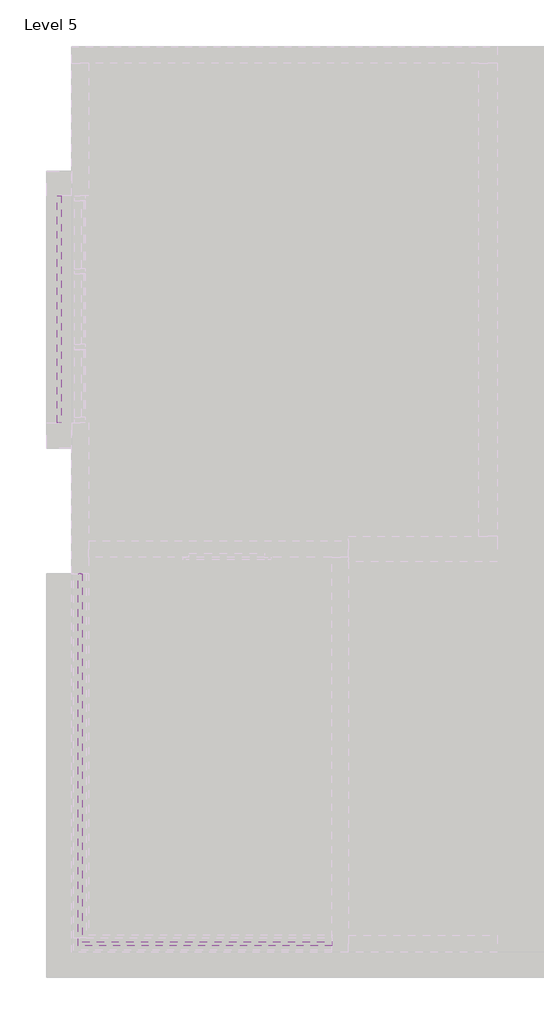
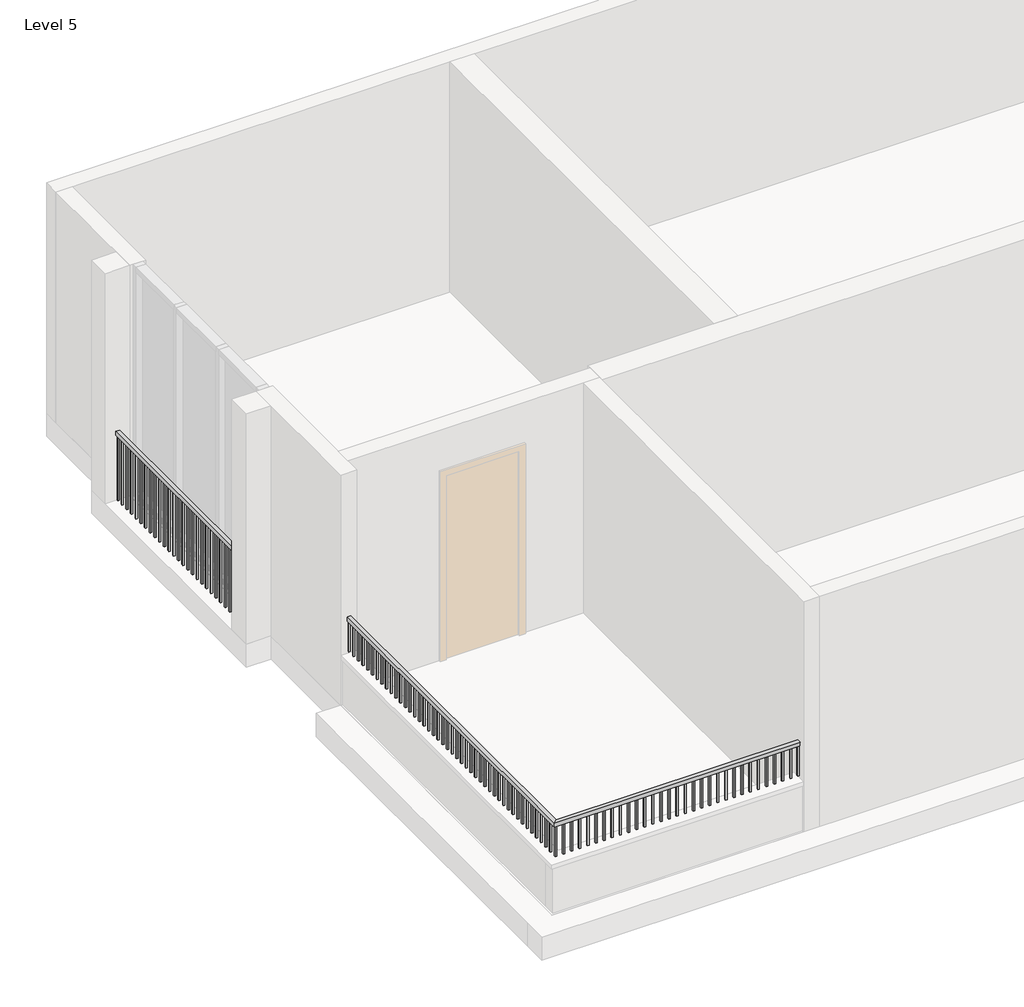
# One storey, part 2 of 2: 2 railings.
"""IFC4 building model written with IfcOpenShell, lengths in millimetres."""

from ifc_helpers import new_model, si_unit, frame, origin, place, context, project, spatial, polyline, outline, extrude, faceted_brep, element, save

model = new_model("IFC4")

# Units and contexts
model_context = context("Model", 3, world=origin())
ifc_project = project(units=[si_unit("LENGTHUNIT", "METRE", prefix="MILLI")], contexts=[model_context])

# Site, building, storey
site = spatial("IfcSite", under=ifc_project)
building = spatial("IfcBuilding", under=site)
storey = spatial("IfcBuildingStorey", under=building, Name="Level 5", Elevation=12192.0)

# Railings
placement = place(None, origin())
element("IfcRailing", 1, ObjectType="Handrail - Rectangular", at=placement, inside=storey, context=model_context, shape_type="SolidModel", body=[
    faceted_brep([(-15179.2169582, -9411.0617616, 14554.2), (-15179.2169582, -9411.0617616, 14503.4), (-15179.2169582, -9360.2617616, 14503.4), (-15179.2169582, -9360.2617616, 14554.2), (-18252.6169582, -9411.0617616, 14554.2), (-18252.6169582, -9411.0617616, 14503.4), (-18201.8169582, -9360.2617616, 14503.4), (-18201.8169582, -9360.2617616, 14554.2), (-18252.6169582, -4908.9117616, 14554.2), (-18201.8169582, -4908.9117616, 14554.2), (-18201.8169582, -4908.9117616, 14503.4), (-18252.6169582, -4908.9117616, 14503.4)], [[[0, 1, 2, 3]], [[1, 0, 4, 5]], [[2, 1, 5, 6]], [[3, 2, 6, 7]], [[0, 3, 7, 4]], [[8, 9, 10, 11]], [[5, 4, 8, 11]], [[6, 5, 11, 10]], [[7, 6, 10, 9]], [[4, 7, 9, 8]]]),
    extrude(outline(polyline([(-18217.6919582, -4924.7867616), (-18236.7419582, -4924.7867616), (-18236.7419582, -4905.7367616), (-18217.6919582, -4905.7367616), (-18217.6919582, -4924.7867616)])), frame((0.0, 0.0, 14097.0), z_axis=(0.0, 0.0, 1.0), x_axis=(1.0, 0.0, 0.0)), (0.0, 0.0, 1.0), 406.4),
    extrude(outline(polyline([(-18217.6919582, -5026.3867616), (-18236.7419582, -5026.3867616), (-18236.7419582, -5007.3367616), (-18217.6919582, -5007.3367616), (-18217.6919582, -5026.3867616)])), frame((0.0, 0.0, 14097.0), z_axis=(0.0, 0.0, 1.0), x_axis=(1.0, 0.0, 0.0)), (0.0, 0.0, 1.0), 406.4),
    extrude(outline(polyline([(-18217.6919582, -5127.9867616), (-18236.7419582, -5127.9867616), (-18236.7419582, -5108.9367616), (-18217.6919582, -5108.9367616), (-18217.6919582, -5127.9867616)])), frame((0.0, 0.0, 14097.0), z_axis=(0.0, 0.0, 1.0), x_axis=(1.0, 0.0, 0.0)), (0.0, 0.0, 1.0), 406.4),
    extrude(outline(polyline([(-18217.6919582, -5229.5867616), (-18236.7419582, -5229.5867616), (-18236.7419582, -5210.5367616), (-18217.6919582, -5210.5367616), (-18217.6919582, -5229.5867616)])), frame((0.0, 0.0, 14097.0), z_axis=(0.0, 0.0, 1.0), x_axis=(1.0, 0.0, 0.0)), (0.0, 0.0, 1.0), 406.4),
    extrude(outline(polyline([(-18217.6919582, -5331.1867616), (-18236.7419582, -5331.1867616), (-18236.7419582, -5312.1367616), (-18217.6919582, -5312.1367616), (-18217.6919582, -5331.1867616)])), frame((0.0, 0.0, 14097.0), z_axis=(0.0, 0.0, 1.0), x_axis=(1.0, 0.0, 0.0)), (0.0, 0.0, 1.0), 406.4),
    extrude(outline(polyline([(-18217.6919582, -5432.7867616), (-18236.7419582, -5432.7867616), (-18236.7419582, -5413.7367616), (-18217.6919582, -5413.7367616), (-18217.6919582, -5432.7867616)])), frame((0.0, 0.0, 14097.0), z_axis=(0.0, 0.0, 1.0), x_axis=(1.0, 0.0, 0.0)), (0.0, 0.0, 1.0), 406.4),
    extrude(outline(polyline([(-18217.6919582, -5534.3867616), (-18236.7419582, -5534.3867616), (-18236.7419582, -5515.3367616), (-18217.6919582, -5515.3367616), (-18217.6919582, -5534.3867616)])), frame((0.0, 0.0, 14097.0), z_axis=(0.0, 0.0, 1.0), x_axis=(1.0, 0.0, 0.0)), (0.0, 0.0, 1.0), 406.4),
    extrude(outline(polyline([(-18217.6919582, -5635.9867616), (-18236.7419582, -5635.9867616), (-18236.7419582, -5616.9367616), (-18217.6919582, -5616.9367616), (-18217.6919582, -5635.9867616)])), frame((0.0, 0.0, 14097.0), z_axis=(0.0, 0.0, 1.0), x_axis=(1.0, 0.0, 0.0)), (0.0, 0.0, 1.0), 406.4),
    extrude(outline(polyline([(-18217.6919582, -5737.5867616), (-18236.7419582, -5737.5867616), (-18236.7419582, -5718.5367616), (-18217.6919582, -5718.5367616), (-18217.6919582, -5737.5867616)])), frame((0.0, 0.0, 14097.0), z_axis=(0.0, 0.0, 1.0), x_axis=(1.0, 0.0, 0.0)), (0.0, 0.0, 1.0), 406.4),
    extrude(outline(polyline([(-18217.6919582, -5839.1867616), (-18236.7419582, -5839.1867616), (-18236.7419582, -5820.1367616), (-18217.6919582, -5820.1367616), (-18217.6919582, -5839.1867616)])), frame((0.0, 0.0, 14097.0), z_axis=(0.0, 0.0, 1.0), x_axis=(1.0, 0.0, 0.0)), (0.0, 0.0, 1.0), 406.4),
    extrude(outline(polyline([(-18217.6919582, -5940.7867616), (-18236.7419582, -5940.7867616), (-18236.7419582, -5921.7367616), (-18217.6919582, -5921.7367616), (-18217.6919582, -5940.7867616)])), frame((0.0, 0.0, 14097.0), z_axis=(0.0, 0.0, 1.0), x_axis=(1.0, 0.0, 0.0)), (0.0, 0.0, 1.0), 406.4),
    extrude(outline(polyline([(-18217.6919582, -6042.3867616), (-18236.7419582, -6042.3867616), (-18236.7419582, -6023.3367616), (-18217.6919582, -6023.3367616), (-18217.6919582, -6042.3867616)])), frame((0.0, 0.0, 14097.0), z_axis=(0.0, 0.0, 1.0), x_axis=(1.0, 0.0, 0.0)), (0.0, 0.0, 1.0), 406.4),
    extrude(outline(polyline([(-18217.6919582, -6143.9867616), (-18236.7419582, -6143.9867616), (-18236.7419582, -6124.9367616), (-18217.6919582, -6124.9367616), (-18217.6919582, -6143.9867616)])), frame((0.0, 0.0, 14097.0), z_axis=(0.0, 0.0, 1.0), x_axis=(1.0, 0.0, 0.0)), (0.0, 0.0, 1.0), 406.4),
    extrude(outline(polyline([(-18217.6919582, -6245.5867616), (-18236.7419582, -6245.5867616), (-18236.7419582, -6226.5367616), (-18217.6919582, -6226.5367616), (-18217.6919582, -6245.5867616)])), frame((0.0, 0.0, 14097.0), z_axis=(0.0, 0.0, 1.0), x_axis=(1.0, 0.0, 0.0)), (0.0, 0.0, 1.0), 406.4),
    extrude(outline(polyline([(-18217.6919582, -6347.1867616), (-18236.7419582, -6347.1867616), (-18236.7419582, -6328.1367616), (-18217.6919582, -6328.1367616), (-18217.6919582, -6347.1867616)])), frame((0.0, 0.0, 14097.0), z_axis=(0.0, 0.0, 1.0), x_axis=(1.0, 0.0, 0.0)), (0.0, 0.0, 1.0), 406.4),
    extrude(outline(polyline([(-18217.6919582, -6448.7867616), (-18236.7419582, -6448.7867616), (-18236.7419582, -6429.7367616), (-18217.6919582, -6429.7367616), (-18217.6919582, -6448.7867616)])), frame((0.0, 0.0, 14097.0), z_axis=(0.0, 0.0, 1.0), x_axis=(1.0, 0.0, 0.0)), (0.0, 0.0, 1.0), 406.4),
    extrude(outline(polyline([(-18217.6919582, -6550.3867616), (-18236.7419582, -6550.3867616), (-18236.7419582, -6531.3367616), (-18217.6919582, -6531.3367616), (-18217.6919582, -6550.3867616)])), frame((0.0, 0.0, 14097.0), z_axis=(0.0, 0.0, 1.0), x_axis=(1.0, 0.0, 0.0)), (0.0, 0.0, 1.0), 406.4),
    extrude(outline(polyline([(-18217.6919582, -6651.9867616), (-18236.7419582, -6651.9867616), (-18236.7419582, -6632.9367616), (-18217.6919582, -6632.9367616), (-18217.6919582, -6651.9867616)])), frame((0.0, 0.0, 14097.0), z_axis=(0.0, 0.0, 1.0), x_axis=(1.0, 0.0, 0.0)), (0.0, 0.0, 1.0), 406.4),
    extrude(outline(polyline([(-18217.6919582, -6753.5867616), (-18236.7419582, -6753.5867616), (-18236.7419582, -6734.5367616), (-18217.6919582, -6734.5367616), (-18217.6919582, -6753.5867616)])), frame((0.0, 0.0, 14097.0), z_axis=(0.0, 0.0, 1.0), x_axis=(1.0, 0.0, 0.0)), (0.0, 0.0, 1.0), 406.4),
    extrude(outline(polyline([(-18217.6919582, -6855.1867616), (-18236.7419582, -6855.1867616), (-18236.7419582, -6836.1367616), (-18217.6919582, -6836.1367616), (-18217.6919582, -6855.1867616)])), frame((0.0, 0.0, 14097.0), z_axis=(0.0, 0.0, 1.0), x_axis=(1.0, 0.0, 0.0)), (0.0, 0.0, 1.0), 406.4),
    extrude(outline(polyline([(-18217.6919582, -6956.7867616), (-18236.7419582, -6956.7867616), (-18236.7419582, -6937.7367616), (-18217.6919582, -6937.7367616), (-18217.6919582, -6956.7867616)])), frame((0.0, 0.0, 14097.0), z_axis=(0.0, 0.0, 1.0), x_axis=(1.0, 0.0, 0.0)), (0.0, 0.0, 1.0), 406.4),
    extrude(outline(polyline([(-18217.6919582, -7058.3867616), (-18236.7419582, -7058.3867616), (-18236.7419582, -7039.3367616), (-18217.6919582, -7039.3367616), (-18217.6919582, -7058.3867616)])), frame((0.0, 0.0, 14097.0), z_axis=(0.0, 0.0, 1.0), x_axis=(1.0, 0.0, 0.0)), (0.0, 0.0, 1.0), 406.4),
    extrude(outline(polyline([(-18217.6919582, -7159.9867616), (-18236.7419582, -7159.9867616), (-18236.7419582, -7140.9367616), (-18217.6919582, -7140.9367616), (-18217.6919582, -7159.9867616)])), frame((0.0, 0.0, 14097.0), z_axis=(0.0, 0.0, 1.0), x_axis=(1.0, 0.0, 0.0)), (0.0, 0.0, 1.0), 406.4),
    extrude(outline(polyline([(-18217.6919582, -7261.5867616), (-18236.7419582, -7261.5867616), (-18236.7419582, -7242.5367616), (-18217.6919582, -7242.5367616), (-18217.6919582, -7261.5867616)])), frame((0.0, 0.0, 14097.0), z_axis=(0.0, 0.0, 1.0), x_axis=(1.0, 0.0, 0.0)), (0.0, 0.0, 1.0), 406.4),
    extrude(outline(polyline([(-18217.6919582, -7363.1867616), (-18236.7419582, -7363.1867616), (-18236.7419582, -7344.1367616), (-18217.6919582, -7344.1367616), (-18217.6919582, -7363.1867616)])), frame((0.0, 0.0, 14097.0), z_axis=(0.0, 0.0, 1.0), x_axis=(1.0, 0.0, 0.0)), (0.0, 0.0, 1.0), 406.4),
    extrude(outline(polyline([(-18217.6919582, -7464.7867616), (-18236.7419582, -7464.7867616), (-18236.7419582, -7445.7367616), (-18217.6919582, -7445.7367616), (-18217.6919582, -7464.7867616)])), frame((0.0, 0.0, 14097.0), z_axis=(0.0, 0.0, 1.0), x_axis=(1.0, 0.0, 0.0)), (0.0, 0.0, 1.0), 406.4),
    extrude(outline(polyline([(-18217.6919582, -7566.3867616), (-18236.7419582, -7566.3867616), (-18236.7419582, -7547.3367616), (-18217.6919582, -7547.3367616), (-18217.6919582, -7566.3867616)])), frame((0.0, 0.0, 14097.0), z_axis=(0.0, 0.0, 1.0), x_axis=(1.0, 0.0, 0.0)), (0.0, 0.0, 1.0), 406.4),
    extrude(outline(polyline([(-18217.6919582, -7667.9867616), (-18236.7419582, -7667.9867616), (-18236.7419582, -7648.9367616), (-18217.6919582, -7648.9367616), (-18217.6919582, -7667.9867616)])), frame((0.0, 0.0, 14097.0), z_axis=(0.0, 0.0, 1.0), x_axis=(1.0, 0.0, 0.0)), (0.0, 0.0, 1.0), 406.4),
    extrude(outline(polyline([(-18217.6919582, -7769.5867616), (-18236.7419582, -7769.5867616), (-18236.7419582, -7750.5367616), (-18217.6919582, -7750.5367616), (-18217.6919582, -7769.5867616)])), frame((0.0, 0.0, 14097.0), z_axis=(0.0, 0.0, 1.0), x_axis=(1.0, 0.0, 0.0)), (0.0, 0.0, 1.0), 406.4),
    extrude(outline(polyline([(-18217.6919582, -7871.1867616), (-18236.7419582, -7871.1867616), (-18236.7419582, -7852.1367616), (-18217.6919582, -7852.1367616), (-18217.6919582, -7871.1867616)])), frame((0.0, 0.0, 14097.0), z_axis=(0.0, 0.0, 1.0), x_axis=(1.0, 0.0, 0.0)), (0.0, 0.0, 1.0), 406.4),
    extrude(outline(polyline([(-18217.6919582, -7972.7867616), (-18236.7419582, -7972.7867616), (-18236.7419582, -7953.7367616), (-18217.6919582, -7953.7367616), (-18217.6919582, -7972.7867616)])), frame((0.0, 0.0, 14097.0), z_axis=(0.0, 0.0, 1.0), x_axis=(1.0, 0.0, 0.0)), (0.0, 0.0, 1.0), 406.4),
    extrude(outline(polyline([(-18217.6919582, -8074.3867616), (-18236.7419582, -8074.3867616), (-18236.7419582, -8055.3367616), (-18217.6919582, -8055.3367616), (-18217.6919582, -8074.3867616)])), frame((0.0, 0.0, 14097.0), z_axis=(0.0, 0.0, 1.0), x_axis=(1.0, 0.0, 0.0)), (0.0, 0.0, 1.0), 406.4),
    extrude(outline(polyline([(-18217.6919582, -8175.9867616), (-18236.7419582, -8175.9867616), (-18236.7419582, -8156.9367616), (-18217.6919582, -8156.9367616), (-18217.6919582, -8175.9867616)])), frame((0.0, 0.0, 14097.0), z_axis=(0.0, 0.0, 1.0), x_axis=(1.0, 0.0, 0.0)), (0.0, 0.0, 1.0), 406.4),
    extrude(outline(polyline([(-18217.6919582, -8277.5867616), (-18236.7419582, -8277.5867616), (-18236.7419582, -8258.5367616), (-18217.6919582, -8258.5367616), (-18217.6919582, -8277.5867616)])), frame((0.0, 0.0, 14097.0), z_axis=(0.0, 0.0, 1.0), x_axis=(1.0, 0.0, 0.0)), (0.0, 0.0, 1.0), 406.4),
    extrude(outline(polyline([(-18217.6919582, -8379.1867616), (-18236.7419582, -8379.1867616), (-18236.7419582, -8360.1367616), (-18217.6919582, -8360.1367616), (-18217.6919582, -8379.1867616)])), frame((0.0, 0.0, 14097.0), z_axis=(0.0, 0.0, 1.0), x_axis=(1.0, 0.0, 0.0)), (0.0, 0.0, 1.0), 406.4),
    extrude(outline(polyline([(-18217.6919582, -8480.7867616), (-18236.7419582, -8480.7867616), (-18236.7419582, -8461.7367616), (-18217.6919582, -8461.7367616), (-18217.6919582, -8480.7867616)])), frame((0.0, 0.0, 14097.0), z_axis=(0.0, 0.0, 1.0), x_axis=(1.0, 0.0, 0.0)), (0.0, 0.0, 1.0), 406.4),
    extrude(outline(polyline([(-18217.6919582, -8582.3867616), (-18236.7419582, -8582.3867616), (-18236.7419582, -8563.3367616), (-18217.6919582, -8563.3367616), (-18217.6919582, -8582.3867616)])), frame((0.0, 0.0, 14097.0), z_axis=(0.0, 0.0, 1.0), x_axis=(1.0, 0.0, 0.0)), (0.0, 0.0, 1.0), 406.4),
    extrude(outline(polyline([(-18217.6919582, -8683.9867616), (-18236.7419582, -8683.9867616), (-18236.7419582, -8664.9367616), (-18217.6919582, -8664.9367616), (-18217.6919582, -8683.9867616)])), frame((0.0, 0.0, 14097.0), z_axis=(0.0, 0.0, 1.0), x_axis=(1.0, 0.0, 0.0)), (0.0, 0.0, 1.0), 406.4),
    extrude(outline(polyline([(-18217.6919582, -8785.5867616), (-18236.7419582, -8785.5867616), (-18236.7419582, -8766.5367616), (-18217.6919582, -8766.5367616), (-18217.6919582, -8785.5867616)])), frame((0.0, 0.0, 14097.0), z_axis=(0.0, 0.0, 1.0), x_axis=(1.0, 0.0, 0.0)), (0.0, 0.0, 1.0), 406.4),
    extrude(outline(polyline([(-18217.6919582, -8887.1867616), (-18236.7419582, -8887.1867616), (-18236.7419582, -8868.1367616), (-18217.6919582, -8868.1367616), (-18217.6919582, -8887.1867616)])), frame((0.0, 0.0, 14097.0), z_axis=(0.0, 0.0, 1.0), x_axis=(1.0, 0.0, 0.0)), (0.0, 0.0, 1.0), 406.4),
    extrude(outline(polyline([(-18217.6919582, -8988.7867616), (-18236.7419582, -8988.7867616), (-18236.7419582, -8969.7367616), (-18217.6919582, -8969.7367616), (-18217.6919582, -8988.7867616)])), frame((0.0, 0.0, 14097.0), z_axis=(0.0, 0.0, 1.0), x_axis=(1.0, 0.0, 0.0)), (0.0, 0.0, 1.0), 406.4),
    extrude(outline(polyline([(-18217.6919582, -9090.3867616), (-18236.7419582, -9090.3867616), (-18236.7419582, -9071.3367616), (-18217.6919582, -9071.3367616), (-18217.6919582, -9090.3867616)])), frame((0.0, 0.0, 14097.0), z_axis=(0.0, 0.0, 1.0), x_axis=(1.0, 0.0, 0.0)), (0.0, 0.0, 1.0), 406.4),
    extrude(outline(polyline([(-18217.6919582, -9191.9867616), (-18236.7419582, -9191.9867616), (-18236.7419582, -9172.9367616), (-18217.6919582, -9172.9367616), (-18217.6919582, -9191.9867616)])), frame((0.0, 0.0, 14097.0), z_axis=(0.0, 0.0, 1.0), x_axis=(1.0, 0.0, 0.0)), (0.0, 0.0, 1.0), 406.4),
    extrude(outline(polyline([(-18217.6919582, -9293.5867616), (-18236.7419582, -9293.5867616), (-18236.7419582, -9274.5367616), (-18217.6919582, -9274.5367616), (-18217.6919582, -9293.5867616)])), frame((0.0, 0.0, 14097.0), z_axis=(0.0, 0.0, 1.0), x_axis=(1.0, 0.0, 0.0)), (0.0, 0.0, 1.0), 406.4),
    extrude(outline(polyline([(-18116.0919582, -9376.1367616), (-18116.0919582, -9395.1867616), (-18135.1419582, -9395.1867616), (-18135.1419582, -9376.1367616), (-18116.0919582, -9376.1367616)])), frame((0.0, 0.0, 14097.0), z_axis=(0.0, 0.0, 1.0), x_axis=(1.0, 0.0, 0.0)), (0.0, 0.0, 1.0), 406.4),
    extrude(outline(polyline([(-18014.4919582, -9376.1367616), (-18014.4919582, -9395.1867616), (-18033.5419582, -9395.1867616), (-18033.5419582, -9376.1367616), (-18014.4919582, -9376.1367616)])), frame((0.0, 0.0, 14097.0), z_axis=(0.0, 0.0, 1.0), x_axis=(1.0, 0.0, 0.0)), (0.0, 0.0, 1.0), 406.4),
    extrude(outline(polyline([(-17912.8919582, -9376.1367616), (-17912.8919582, -9395.1867616), (-17931.9419582, -9395.1867616), (-17931.9419582, -9376.1367616), (-17912.8919582, -9376.1367616)])), frame((0.0, 0.0, 14097.0), z_axis=(0.0, 0.0, 1.0), x_axis=(1.0, 0.0, 0.0)), (0.0, 0.0, 1.0), 406.4),
    extrude(outline(polyline([(-17811.2919582, -9376.1367616), (-17811.2919582, -9395.1867616), (-17830.3419582, -9395.1867616), (-17830.3419582, -9376.1367616), (-17811.2919582, -9376.1367616)])), frame((0.0, 0.0, 14097.0), z_axis=(0.0, 0.0, 1.0), x_axis=(1.0, 0.0, 0.0)), (0.0, 0.0, 1.0), 406.4),
    extrude(outline(polyline([(-17709.6919582, -9376.1367616), (-17709.6919582, -9395.1867616), (-17728.7419582, -9395.1867616), (-17728.7419582, -9376.1367616), (-17709.6919582, -9376.1367616)])), frame((0.0, 0.0, 14097.0), z_axis=(0.0, 0.0, 1.0), x_axis=(1.0, 0.0, 0.0)), (0.0, 0.0, 1.0), 406.4),
    extrude(outline(polyline([(-17608.0919582, -9376.1367616), (-17608.0919582, -9395.1867616), (-17627.1419582, -9395.1867616), (-17627.1419582, -9376.1367616), (-17608.0919582, -9376.1367616)])), frame((0.0, 0.0, 14097.0), z_axis=(0.0, 0.0, 1.0), x_axis=(1.0, 0.0, 0.0)), (0.0, 0.0, 1.0), 406.4),
    extrude(outline(polyline([(-17506.4919582, -9376.1367616), (-17506.4919582, -9395.1867616), (-17525.5419582, -9395.1867616), (-17525.5419582, -9376.1367616), (-17506.4919582, -9376.1367616)])), frame((0.0, 0.0, 14097.0), z_axis=(0.0, 0.0, 1.0), x_axis=(1.0, 0.0, 0.0)), (0.0, 0.0, 1.0), 406.4),
    extrude(outline(polyline([(-17404.8919582, -9376.1367616), (-17404.8919582, -9395.1867616), (-17423.9419582, -9395.1867616), (-17423.9419582, -9376.1367616), (-17404.8919582, -9376.1367616)])), frame((0.0, 0.0, 14097.0), z_axis=(0.0, 0.0, 1.0), x_axis=(1.0, 0.0, 0.0)), (0.0, 0.0, 1.0), 406.4),
    extrude(outline(polyline([(-17303.2919582, -9376.1367616), (-17303.2919582, -9395.1867616), (-17322.3419582, -9395.1867616), (-17322.3419582, -9376.1367616), (-17303.2919582, -9376.1367616)])), frame((0.0, 0.0, 14097.0), z_axis=(0.0, 0.0, 1.0), x_axis=(1.0, 0.0, 0.0)), (0.0, 0.0, 1.0), 406.4),
    extrude(outline(polyline([(-17201.6919582, -9376.1367616), (-17201.6919582, -9395.1867616), (-17220.7419582, -9395.1867616), (-17220.7419582, -9376.1367616), (-17201.6919582, -9376.1367616)])), frame((0.0, 0.0, 14097.0), z_axis=(0.0, 0.0, 1.0), x_axis=(1.0, 0.0, 0.0)), (0.0, 0.0, 1.0), 406.4),
    extrude(outline(polyline([(-17100.0919582, -9376.1367616), (-17100.0919582, -9395.1867616), (-17119.1419582, -9395.1867616), (-17119.1419582, -9376.1367616), (-17100.0919582, -9376.1367616)])), frame((0.0, 0.0, 14097.0), z_axis=(0.0, 0.0, 1.0), x_axis=(1.0, 0.0, 0.0)), (0.0, 0.0, 1.0), 406.4),
    extrude(outline(polyline([(-16998.4919582, -9376.1367616), (-16998.4919582, -9395.1867616), (-17017.5419582, -9395.1867616), (-17017.5419582, -9376.1367616), (-16998.4919582, -9376.1367616)])), frame((0.0, 0.0, 14097.0), z_axis=(0.0, 0.0, 1.0), x_axis=(1.0, 0.0, 0.0)), (0.0, 0.0, 1.0), 406.4),
    extrude(outline(polyline([(-16896.8919582, -9376.1367616), (-16896.8919582, -9395.1867616), (-16915.9419582, -9395.1867616), (-16915.9419582, -9376.1367616), (-16896.8919582, -9376.1367616)])), frame((0.0, 0.0, 14097.0), z_axis=(0.0, 0.0, 1.0), x_axis=(1.0, 0.0, 0.0)), (0.0, 0.0, 1.0), 406.4),
    extrude(outline(polyline([(-16795.2919582, -9376.1367616), (-16795.2919582, -9395.1867616), (-16814.3419582, -9395.1867616), (-16814.3419582, -9376.1367616), (-16795.2919582, -9376.1367616)])), frame((0.0, 0.0, 14097.0), z_axis=(0.0, 0.0, 1.0), x_axis=(1.0, 0.0, 0.0)), (0.0, 0.0, 1.0), 406.4),
    extrude(outline(polyline([(-16693.6919582, -9376.1367616), (-16693.6919582, -9395.1867616), (-16712.7419582, -9395.1867616), (-16712.7419582, -9376.1367616), (-16693.6919582, -9376.1367616)])), frame((0.0, 0.0, 14097.0), z_axis=(0.0, 0.0, 1.0), x_axis=(1.0, 0.0, 0.0)), (0.0, 0.0, 1.0), 406.4),
    extrude(outline(polyline([(-16592.0919582, -9376.1367616), (-16592.0919582, -9395.1867616), (-16611.1419582, -9395.1867616), (-16611.1419582, -9376.1367616), (-16592.0919582, -9376.1367616)])), frame((0.0, 0.0, 14097.0), z_axis=(0.0, 0.0, 1.0), x_axis=(1.0, 0.0, 0.0)), (0.0, 0.0, 1.0), 406.4),
    extrude(outline(polyline([(-16490.4919582, -9376.1367616), (-16490.4919582, -9395.1867616), (-16509.5419582, -9395.1867616), (-16509.5419582, -9376.1367616), (-16490.4919582, -9376.1367616)])), frame((0.0, 0.0, 14097.0), z_axis=(0.0, 0.0, 1.0), x_axis=(1.0, 0.0, 0.0)), (0.0, 0.0, 1.0), 406.4),
    extrude(outline(polyline([(-16388.8919582, -9376.1367616), (-16388.8919582, -9395.1867616), (-16407.9419582, -9395.1867616), (-16407.9419582, -9376.1367616), (-16388.8919582, -9376.1367616)])), frame((0.0, 0.0, 14097.0), z_axis=(0.0, 0.0, 1.0), x_axis=(1.0, 0.0, 0.0)), (0.0, 0.0, 1.0), 406.4),
    extrude(outline(polyline([(-16287.2919582, -9376.1367616), (-16287.2919582, -9395.1867616), (-16306.3419582, -9395.1867616), (-16306.3419582, -9376.1367616), (-16287.2919582, -9376.1367616)])), frame((0.0, 0.0, 14097.0), z_axis=(0.0, 0.0, 1.0), x_axis=(1.0, 0.0, 0.0)), (0.0, 0.0, 1.0), 406.4),
    extrude(outline(polyline([(-16185.6919582, -9376.1367616), (-16185.6919582, -9395.1867616), (-16204.7419582, -9395.1867616), (-16204.7419582, -9376.1367616), (-16185.6919582, -9376.1367616)])), frame((0.0, 0.0, 14097.0), z_axis=(0.0, 0.0, 1.0), x_axis=(1.0, 0.0, 0.0)), (0.0, 0.0, 1.0), 406.4),
    extrude(outline(polyline([(-16084.0919582, -9376.1367616), (-16084.0919582, -9395.1867616), (-16103.1419582, -9395.1867616), (-16103.1419582, -9376.1367616), (-16084.0919582, -9376.1367616)])), frame((0.0, 0.0, 14097.0), z_axis=(0.0, 0.0, 1.0), x_axis=(1.0, 0.0, 0.0)), (0.0, 0.0, 1.0), 406.4),
    extrude(outline(polyline([(-15982.4919582, -9376.1367616), (-15982.4919582, -9395.1867616), (-16001.5419582, -9395.1867616), (-16001.5419582, -9376.1367616), (-15982.4919582, -9376.1367616)])), frame((0.0, 0.0, 14097.0), z_axis=(0.0, 0.0, 1.0), x_axis=(1.0, 0.0, 0.0)), (0.0, 0.0, 1.0), 406.4),
    extrude(outline(polyline([(-15880.8919582, -9376.1367616), (-15880.8919582, -9395.1867616), (-15899.9419582, -9395.1867616), (-15899.9419582, -9376.1367616), (-15880.8919582, -9376.1367616)])), frame((0.0, 0.0, 14097.0), z_axis=(0.0, 0.0, 1.0), x_axis=(1.0, 0.0, 0.0)), (0.0, 0.0, 1.0), 406.4),
    extrude(outline(polyline([(-15779.2919582, -9376.1367616), (-15779.2919582, -9395.1867616), (-15798.3419582, -9395.1867616), (-15798.3419582, -9376.1367616), (-15779.2919582, -9376.1367616)])), frame((0.0, 0.0, 14097.0), z_axis=(0.0, 0.0, 1.0), x_axis=(1.0, 0.0, 0.0)), (0.0, 0.0, 1.0), 406.4),
    extrude(outline(polyline([(-15677.6919582, -9376.1367616), (-15677.6919582, -9395.1867616), (-15696.7419582, -9395.1867616), (-15696.7419582, -9376.1367616), (-15677.6919582, -9376.1367616)])), frame((0.0, 0.0, 14097.0), z_axis=(0.0, 0.0, 1.0), x_axis=(1.0, 0.0, 0.0)), (0.0, 0.0, 1.0), 406.4),
    extrude(outline(polyline([(-15576.0919582, -9376.1367616), (-15576.0919582, -9395.1867616), (-15595.1419582, -9395.1867616), (-15595.1419582, -9376.1367616), (-15576.0919582, -9376.1367616)])), frame((0.0, 0.0, 14097.0), z_axis=(0.0, 0.0, 1.0), x_axis=(1.0, 0.0, 0.0)), (0.0, 0.0, 1.0), 406.4),
    extrude(outline(polyline([(-15474.4919582, -9376.1367616), (-15474.4919582, -9395.1867616), (-15493.5419582, -9395.1867616), (-15493.5419582, -9376.1367616), (-15474.4919582, -9376.1367616)])), frame((0.0, 0.0, 14097.0), z_axis=(0.0, 0.0, 1.0), x_axis=(1.0, 0.0, 0.0)), (0.0, 0.0, 1.0), 406.4),
    extrude(outline(polyline([(-15372.8919582, -9376.1367616), (-15372.8919582, -9395.1867616), (-15391.9419582, -9395.1867616), (-15391.9419582, -9376.1367616), (-15372.8919582, -9376.1367616)])), frame((0.0, 0.0, 14097.0), z_axis=(0.0, 0.0, 1.0), x_axis=(1.0, 0.0, 0.0)), (0.0, 0.0, 1.0), 406.4),
    extrude(outline(polyline([(-15271.2919582, -9376.1367616), (-15271.2919582, -9395.1867616), (-15290.3419582, -9395.1867616), (-15290.3419582, -9376.1367616), (-15271.2919582, -9376.1367616)])), frame((0.0, 0.0, 14097.0), z_axis=(0.0, 0.0, 1.0), x_axis=(1.0, 0.0, 0.0)), (0.0, 0.0, 1.0), 406.4),
    extrude(outline(polyline([(-18217.6919582, -9376.1367616), (-18217.6919582, -9395.1867616), (-18236.7419582, -9395.1867616), (-18236.7419582, -9376.1367616), (-18217.6919582, -9376.1367616)])), frame((0.0, 0.0, 14097.0), z_axis=(0.0, 0.0, 1.0), x_axis=(1.0, 0.0, 0.0)), (0.0, 0.0, 1.0), 406.4),
    extrude(outline(polyline([(-18217.6919582, -4927.9617616), (-18236.7419582, -4927.9617616), (-18236.7419582, -4908.9117616), (-18217.6919582, -4908.9117616), (-18217.6919582, -4927.9617616)])), frame((0.0, 0.0, 14097.0), z_axis=(0.0, 0.0, 1.0), x_axis=(1.0, 0.0, 0.0)), (0.0, 0.0, 1.0), 406.4),
    extrude(outline(polyline([(-15179.2169582, -9376.1367616), (-15179.2169582, -9395.1867616), (-15198.2669582, -9395.1867616), (-15198.2669582, -9376.1367616), (-15179.2169582, -9376.1367616)])), frame((0.0, 0.0, 14097.0), z_axis=(0.0, 0.0, 1.0), x_axis=(1.0, 0.0, 0.0)), (0.0, 0.0, 1.0), 406.4),
])
element("IfcRailing", 2, ObjectType="Handrail - Rectangular 2", at=placement, inside=storey, context=model_context, shape_type="SweptSolid", body=[
    extrude(outline(polyline([(-18506.6169582, -336.9117616), (-18455.8169582, -336.9117616), (-18455.8169582, -3080.1117616), (-18506.6169582, -3080.1117616), (-18506.6169582, -336.9117616)])), frame((0.0, 0.0, 14274.8), z_axis=(0.0, 0.0, 1.0), x_axis=(1.0, 0.0, 0.0)), (0.0, 0.0, 1.0), 50.8),
    extrude(outline(polyline([(-18490.7419582, -2968.9867616), (-18471.6919582, -2968.9867616), (-18471.6919582, -2988.0367616), (-18490.7419582, -2988.0367616), (-18490.7419582, -2968.9867616)])), frame((0.0, 0.0, 13411.2), z_axis=(0.0, 0.0, 1.0), x_axis=(1.0, 0.0, 0.0)), (0.0, 0.0, 1.0), 863.6),
    extrude(outline(polyline([(-18490.7419582, -2867.3867616), (-18471.6919582, -2867.3867616), (-18471.6919582, -2886.4367616), (-18490.7419582, -2886.4367616), (-18490.7419582, -2867.3867616)])), frame((0.0, 0.0, 13411.2), z_axis=(0.0, 0.0, 1.0), x_axis=(1.0, 0.0, 0.0)), (0.0, 0.0, 1.0), 863.6),
    extrude(outline(polyline([(-18490.7419582, -2765.7867616), (-18471.6919582, -2765.7867616), (-18471.6919582, -2784.8367616), (-18490.7419582, -2784.8367616), (-18490.7419582, -2765.7867616)])), frame((0.0, 0.0, 13411.2), z_axis=(0.0, 0.0, 1.0), x_axis=(1.0, 0.0, 0.0)), (0.0, 0.0, 1.0), 863.6),
    extrude(outline(polyline([(-18490.7419582, -2664.1867616), (-18471.6919582, -2664.1867616), (-18471.6919582, -2683.2367616), (-18490.7419582, -2683.2367616), (-18490.7419582, -2664.1867616)])), frame((0.0, 0.0, 13411.2), z_axis=(0.0, 0.0, 1.0), x_axis=(1.0, 0.0, 0.0)), (0.0, 0.0, 1.0), 863.6),
    extrude(outline(polyline([(-18490.7419582, -2562.5867616), (-18471.6919582, -2562.5867616), (-18471.6919582, -2581.6367616), (-18490.7419582, -2581.6367616), (-18490.7419582, -2562.5867616)])), frame((0.0, 0.0, 13411.2), z_axis=(0.0, 0.0, 1.0), x_axis=(1.0, 0.0, 0.0)), (0.0, 0.0, 1.0), 863.6),
    extrude(outline(polyline([(-18490.7419582, -2460.9867616), (-18471.6919582, -2460.9867616), (-18471.6919582, -2480.0367616), (-18490.7419582, -2480.0367616), (-18490.7419582, -2460.9867616)])), frame((0.0, 0.0, 13411.2), z_axis=(0.0, 0.0, 1.0), x_axis=(1.0, 0.0, 0.0)), (0.0, 0.0, 1.0), 863.6),
    extrude(outline(polyline([(-18490.7419582, -2359.3867616), (-18471.6919582, -2359.3867616), (-18471.6919582, -2378.4367616), (-18490.7419582, -2378.4367616), (-18490.7419582, -2359.3867616)])), frame((0.0, 0.0, 13411.2), z_axis=(0.0, 0.0, 1.0), x_axis=(1.0, 0.0, 0.0)), (0.0, 0.0, 1.0), 863.6),
    extrude(outline(polyline([(-18490.7419582, -2257.7867616), (-18471.6919582, -2257.7867616), (-18471.6919582, -2276.8367616), (-18490.7419582, -2276.8367616), (-18490.7419582, -2257.7867616)])), frame((0.0, 0.0, 13411.2), z_axis=(0.0, 0.0, 1.0), x_axis=(1.0, 0.0, 0.0)), (0.0, 0.0, 1.0), 863.6),
    extrude(outline(polyline([(-18490.7419582, -2156.1867616), (-18471.6919582, -2156.1867616), (-18471.6919582, -2175.2367616), (-18490.7419582, -2175.2367616), (-18490.7419582, -2156.1867616)])), frame((0.0, 0.0, 13411.2), z_axis=(0.0, 0.0, 1.0), x_axis=(1.0, 0.0, 0.0)), (0.0, 0.0, 1.0), 863.6),
    extrude(outline(polyline([(-18490.7419582, -2054.5867616), (-18471.6919582, -2054.5867616), (-18471.6919582, -2073.6367616), (-18490.7419582, -2073.6367616), (-18490.7419582, -2054.5867616)])), frame((0.0, 0.0, 13411.2), z_axis=(0.0, 0.0, 1.0), x_axis=(1.0, 0.0, 0.0)), (0.0, 0.0, 1.0), 863.6),
    extrude(outline(polyline([(-18490.7419582, -1952.9867616), (-18471.6919582, -1952.9867616), (-18471.6919582, -1972.0367616), (-18490.7419582, -1972.0367616), (-18490.7419582, -1952.9867616)])), frame((0.0, 0.0, 13411.2), z_axis=(0.0, 0.0, 1.0), x_axis=(1.0, 0.0, 0.0)), (0.0, 0.0, 1.0), 863.6),
    extrude(outline(polyline([(-18490.7419582, -1851.3867616), (-18471.6919582, -1851.3867616), (-18471.6919582, -1870.4367616), (-18490.7419582, -1870.4367616), (-18490.7419582, -1851.3867616)])), frame((0.0, 0.0, 13411.2), z_axis=(0.0, 0.0, 1.0), x_axis=(1.0, 0.0, 0.0)), (0.0, 0.0, 1.0), 863.6),
    extrude(outline(polyline([(-18490.7419582, -1749.7867616), (-18471.6919582, -1749.7867616), (-18471.6919582, -1768.8367616), (-18490.7419582, -1768.8367616), (-18490.7419582, -1749.7867616)])), frame((0.0, 0.0, 13411.2), z_axis=(0.0, 0.0, 1.0), x_axis=(1.0, 0.0, 0.0)), (0.0, 0.0, 1.0), 863.6),
    extrude(outline(polyline([(-18490.7419582, -1648.1867616), (-18471.6919582, -1648.1867616), (-18471.6919582, -1667.2367616), (-18490.7419582, -1667.2367616), (-18490.7419582, -1648.1867616)])), frame((0.0, 0.0, 13411.2), z_axis=(0.0, 0.0, 1.0), x_axis=(1.0, 0.0, 0.0)), (0.0, 0.0, 1.0), 863.6),
    extrude(outline(polyline([(-18490.7419582, -1546.5867616), (-18471.6919582, -1546.5867616), (-18471.6919582, -1565.6367616), (-18490.7419582, -1565.6367616), (-18490.7419582, -1546.5867616)])), frame((0.0, 0.0, 13411.2), z_axis=(0.0, 0.0, 1.0), x_axis=(1.0, 0.0, 0.0)), (0.0, 0.0, 1.0), 863.6),
    extrude(outline(polyline([(-18490.7419582, -1444.9867616), (-18471.6919582, -1444.9867616), (-18471.6919582, -1464.0367616), (-18490.7419582, -1464.0367616), (-18490.7419582, -1444.9867616)])), frame((0.0, 0.0, 13411.2), z_axis=(0.0, 0.0, 1.0), x_axis=(1.0, 0.0, 0.0)), (0.0, 0.0, 1.0), 863.6),
    extrude(outline(polyline([(-18490.7419582, -1343.3867616), (-18471.6919582, -1343.3867616), (-18471.6919582, -1362.4367616), (-18490.7419582, -1362.4367616), (-18490.7419582, -1343.3867616)])), frame((0.0, 0.0, 13411.2), z_axis=(0.0, 0.0, 1.0), x_axis=(1.0, 0.0, 0.0)), (0.0, 0.0, 1.0), 863.6),
    extrude(outline(polyline([(-18490.7419582, -1241.7867616), (-18471.6919582, -1241.7867616), (-18471.6919582, -1260.8367616), (-18490.7419582, -1260.8367616), (-18490.7419582, -1241.7867616)])), frame((0.0, 0.0, 13411.2), z_axis=(0.0, 0.0, 1.0), x_axis=(1.0, 0.0, 0.0)), (0.0, 0.0, 1.0), 863.6),
    extrude(outline(polyline([(-18490.7419582, -1140.1867616), (-18471.6919582, -1140.1867616), (-18471.6919582, -1159.2367616), (-18490.7419582, -1159.2367616), (-18490.7419582, -1140.1867616)])), frame((0.0, 0.0, 13411.2), z_axis=(0.0, 0.0, 1.0), x_axis=(1.0, 0.0, 0.0)), (0.0, 0.0, 1.0), 863.6),
    extrude(outline(polyline([(-18490.7419582, -1038.5867616), (-18471.6919582, -1038.5867616), (-18471.6919582, -1057.6367616), (-18490.7419582, -1057.6367616), (-18490.7419582, -1038.5867616)])), frame((0.0, 0.0, 13411.2), z_axis=(0.0, 0.0, 1.0), x_axis=(1.0, 0.0, 0.0)), (0.0, 0.0, 1.0), 863.6),
    extrude(outline(polyline([(-18490.7419582, -936.9867616), (-18471.6919582, -936.9867616), (-18471.6919582, -956.0367616), (-18490.7419582, -956.0367616), (-18490.7419582, -936.9867616)])), frame((0.0, 0.0, 13411.2), z_axis=(0.0, 0.0, 1.0), x_axis=(1.0, 0.0, 0.0)), (0.0, 0.0, 1.0), 863.6),
    extrude(outline(polyline([(-18490.7419582, -835.3867616), (-18471.6919582, -835.3867616), (-18471.6919582, -854.4367616), (-18490.7419582, -854.4367616), (-18490.7419582, -835.3867616)])), frame((0.0, 0.0, 13411.2), z_axis=(0.0, 0.0, 1.0), x_axis=(1.0, 0.0, 0.0)), (0.0, 0.0, 1.0), 863.6),
    extrude(outline(polyline([(-18490.7419582, -733.7867616), (-18471.6919582, -733.7867616), (-18471.6919582, -752.8367616), (-18490.7419582, -752.8367616), (-18490.7419582, -733.7867616)])), frame((0.0, 0.0, 13411.2), z_axis=(0.0, 0.0, 1.0), x_axis=(1.0, 0.0, 0.0)), (0.0, 0.0, 1.0), 863.6),
    extrude(outline(polyline([(-18490.7419582, -632.1867616), (-18471.6919582, -632.1867616), (-18471.6919582, -651.2367616), (-18490.7419582, -651.2367616), (-18490.7419582, -632.1867616)])), frame((0.0, 0.0, 13411.2), z_axis=(0.0, 0.0, 1.0), x_axis=(1.0, 0.0, 0.0)), (0.0, 0.0, 1.0), 863.6),
    extrude(outline(polyline([(-18490.7419582, -530.5867616), (-18471.6919582, -530.5867616), (-18471.6919582, -549.6367616), (-18490.7419582, -549.6367616), (-18490.7419582, -530.5867616)])), frame((0.0, 0.0, 13411.2), z_axis=(0.0, 0.0, 1.0), x_axis=(1.0, 0.0, 0.0)), (0.0, 0.0, 1.0), 863.6),
    extrude(outline(polyline([(-18490.7419582, -428.9867616), (-18471.6919582, -428.9867616), (-18471.6919582, -448.0367616), (-18490.7419582, -448.0367616), (-18490.7419582, -428.9867616)])), frame((0.0, 0.0, 13411.2), z_axis=(0.0, 0.0, 1.0), x_axis=(1.0, 0.0, 0.0)), (0.0, 0.0, 1.0), 863.6),
    extrude(outline(polyline([(-18490.7419582, -3061.0617616), (-18471.6919582, -3061.0617616), (-18471.6919582, -3080.1117616), (-18490.7419582, -3080.1117616), (-18490.7419582, -3061.0617616)])), frame((0.0, 0.0, 13411.2), z_axis=(0.0, 0.0, 1.0), x_axis=(1.0, 0.0, 0.0)), (0.0, 0.0, 1.0), 863.6),
    extrude(outline(polyline([(-18490.7419582, -336.9117616), (-18471.6919582, -336.9117616), (-18471.6919582, -355.9617616), (-18490.7419582, -355.9617616), (-18490.7419582, -336.9117616)])), frame((0.0, 0.0, 13411.2), z_axis=(0.0, 0.0, 1.0), x_axis=(1.0, 0.0, 0.0)), (0.0, 0.0, 1.0), 863.6),
])

save(model, "model.ifc")

# Revit data of these elements
# Type "Handrail - Rectangular"
#   Assembly Code = "C2010400"
#   built-in parameter 1008612 = 0.0416667 (stored number, unit not read)
#   built-in parameter 1008611 = 0.0416667 (stored number, unit not read)
#   built-in parameter 1008609 = 0.333333 (stored number, unit not read)
#   built-in parameter 1008604 = 0.166667 (stored number, unit not read)
#   built-in parameter 1008603 = 0.166667 (stored number, unit not read)
#   Railing Height = 1' - 6"
#   built-in parameter 1008630 = 2
#   built-in parameter 1008610 = 2
#   built-in parameter 1008618 = Baluster - Square : 3/4"
# Type "Handrail - Rectangular 2"
#   Assembly Code = "C2010400"
#   built-in parameter 1008612 = 0.0416667 (stored number, unit not read)
#   built-in parameter 1008611 = 0.0416667 (stored number, unit not read)
#   built-in parameter 1008609 = 0.333333 (stored number, unit not read)
#   built-in parameter 1008604 = 0.166667 (stored number, unit not read)
#   built-in parameter 1008603 = 0.166667 (stored number, unit not read)
#   Railing Height = 3' - 0"
#   built-in parameter 1008630 = 2
#   built-in parameter 1008610 = 2
#   built-in parameter 1008618 = Baluster - Square : 3/4"
# Element 1 (IfcRailing, "Handrail - Rectangular")
#   built-in parameter 1008621 = 6.25 (stored number, unit not read)
#   Phase Created = New Construction
# Element 2 (IfcRailing, "Handrail - Rectangular 2")
#   built-in parameter 1008621 = 4 (stored number, unit not read)
#   Phase Created = New Construction
